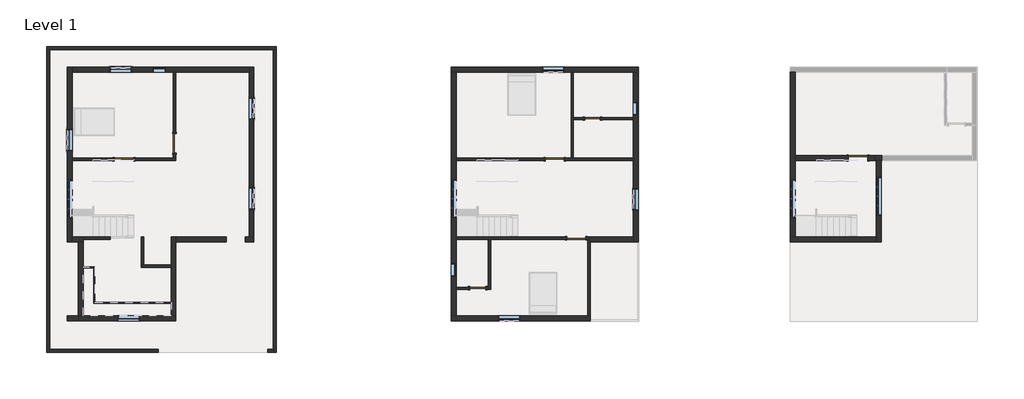
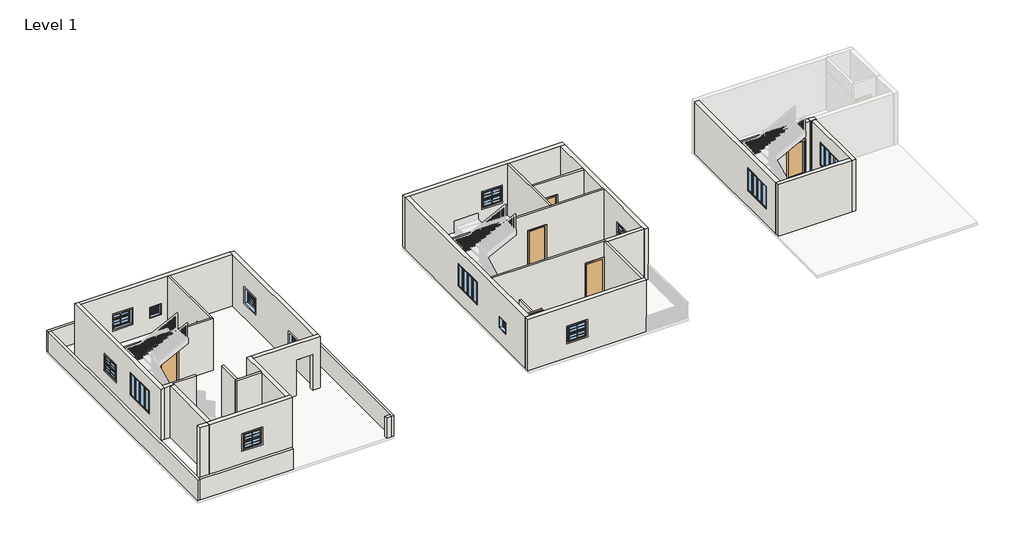
# One storey, part 1 of 8: 40 walls, 15 windows, 7 doors.
"""IFC4 building model written with IfcOpenShell, lengths in millimetres."""

from ifc_helpers import new_model, si_unit, frame, origin, origin_with_axes, place, context, project, spatial, polyline, outline, extrude, faceted_brep, transform, mapped, element, save
from components import door_f2b275c1, door_d8f5dbb5, single_flush_door_3_17d80c48, single_flush_door_3_5e62189b, single_flush_door_3_89fc3733, window_fa0038f5, window_5487fb6d, window_f2d8fef0

model = new_model("IFC4")

# Units and contexts
model_context = context("Model", 3, world=origin())
ifc_project = project(units=[si_unit("LENGTHUNIT", "METRE", prefix="MILLI")], contexts=[model_context])

# Site, building, storey
site = spatial("IfcSite", under=ifc_project)
building = spatial("IfcBuilding", under=site)
storey = spatial("IfcBuildingStorey", under=building, Name="Level 1", Elevation=0.0)

# Doors
placement = place(None, origin())
door_shape = door_f2b275c1(model_context)
element("IfcDoor", 1, ObjectType="Single-Flush : door 2'6\"", at=placement, inside=storey, context=model_context, shape_type="MappedRepresentation", body=[
    mapped(door_shape, transform((2134.2191518, 4539.4100713, 0.0), x_axis=(-1.0, 0.0, 0.0), y_axis=(0.0, -1.0, 0.0), z_axis=(0.0, 0.0, 1.0))),
])
door_2_shape = door_d8f5dbb5(model_context)
element("IfcDoor", 2, ObjectType="Single-Flush : door 2'6\"", at=placement, inside=storey, context=model_context, shape_type="MappedRepresentation", body=[
    mapped(door_2_shape, transform((-3352.1808482, -3575.8899287, 0.0), x_axis=(1.0, 0.0, 0.0), y_axis=(0.0, 1.0, 0.0), z_axis=(0.0, 0.0, 1.0))),
])
single_flush_door_3_shape = single_flush_door_3_17d80c48(model_context)
element("IfcDoor", 3, ObjectType="Single-Flush : door 3'", at=placement, inside=storey, context=model_context, shape_type="MappedRepresentation", body=[
    mapped(single_flush_door_3_shape, transform((-20233.4289184, 2596.3100713, 0.0), x_axis=(1.0, 0.0, 0.0), y_axis=(0.0, 1.0, 0.0), z_axis=(0.0, 0.0, 1.0))),
])
element("IfcDoor", 4, ObjectType="Single-Flush : door 3'", at=placement, inside=storey, context=model_context, shape_type="MappedRepresentation", body=[
    mapped(single_flush_door_3_shape, transform((330.8191518, 2596.3100713, 0.0), x_axis=(1.0, 0.0, 0.0), y_axis=(0.0, 1.0, 0.0), z_axis=(0.0, 0.0, 1.0))),
])
single_flush_door_3_2_shape = single_flush_door_3_5e62189b(model_context)
element("IfcDoor", 5, ObjectType="Single-Flush : door 3'", at=placement, inside=storey, context=model_context, shape_type="MappedRepresentation", body=[
    mapped(single_flush_door_3_2_shape, transform((-17820.4289184, 3358.3100713, 0.0), x_axis=(0.0, -1.0, 0.0), y_axis=(1.0, 0.0, 0.0), z_axis=(0.0, 0.0, 1.0))),
])
element("IfcDoor", 6, ObjectType="Single-Flush : door 3'", at=placement, inside=storey, context=model_context, shape_type="MappedRepresentation", body=[
    mapped(single_flush_door_3_2_shape, transform((1359.5191518, -1175.5899287, 0.0), x_axis=(1.0, 0.0, 0.0), y_axis=(0.0, 1.0, 0.0), z_axis=(0.0, 0.0, 1.0))),
])
single_flush_door_3_3_shape = single_flush_door_3_89fc3733(model_context)
element("IfcDoor", 7, ObjectType="Single-Flush : door 3'", at=placement, inside=storey, context=model_context, shape_type="MappedRepresentation", body=[
    mapped(single_flush_door_3_3_shape, transform((14813.742447, 2653.4600713, 0.0), x_axis=(1.0, 0.0, 0.0), y_axis=(0.0, 1.0, 0.0), z_axis=(0.0, 0.0, 1.0))),
])

# Walls
element("IfcWall", 8, at=placement, inside=storey, context=model_context, shape_type="Brep", body=[
    faceted_brep([(-23935.4789184, 7835.0600713, 0.0), (-23783.0789184, 7835.0600713, 0.0), (-13115.0789184, 7835.0600713, 0.0), (-12962.6789184, 7835.0600713, 0.0), (-12962.6789184, 7835.0600713, 1219.2), (-13115.0789184, 7835.0600713, 1219.2), (-23783.0789184, 7835.0600713, 1219.2), (-23935.4789184, 7835.0600713, 1219.2), (-23935.4789184, 7987.4600713, 0.0), (-23935.4789184, 7987.4600713, 1219.2), (-12962.6789184, 7987.4600713, 1219.2), (-12962.6789184, 7987.4600713, 0.0)], [[[0, 1, 2, 3, 4, 5, 6, 7]], [[8, 9, 10, 11]], [[3, 2, 1, 0, 8, 11]], [[7, 6, 5, 4, 10, 9]], [[4, 3, 11, 10]], [[0, 7, 9, 8]]]),
])
element("IfcWall", 9, at=placement, inside=storey, context=model_context, shape_type="Brep", body=[
    faceted_brep([(-13115.0789184, 7835.0600713, 0.0), (-13115.0789184, -6490.5399287, 0.0), (-13115.0789184, -6642.9399287, 0.0), (-13115.0789184, -6642.9399287, 1219.2), (-13115.0789184, -6490.5399287, 1219.2), (-13115.0789184, 7835.0600713, 1219.2), (-12962.6789184, 7835.0600713, 0.0), (-12962.6789184, 7835.0600713, 1219.2), (-12962.6789184, -6642.9399287, 1219.2), (-12962.6789184, -6642.9399287, 0.0)], [[[0, 1, 2, 3, 4, 5]], [[6, 7, 8, 9]], [[2, 1, 0, 6, 9]], [[5, 4, 3, 8, 7]], [[0, 5, 7, 6]], [[3, 2, 9, 8]]]),
])
element("IfcWall", 10, at=placement, inside=storey, context=model_context, shape_type="Brep", body=[
    faceted_brep([(-23935.4789184, 7835.0600713, 0.0), (-23935.4789184, -6642.9399287, 0.0), (-23935.4789184, -6642.9399287, 1219.2), (-23935.4789184, 7835.0600713, 1219.2), (-23783.0789184, 7835.0600713, 0.0), (-23783.0789184, 7835.0600713, 1219.2), (-23783.0789184, -6490.5399287, 1219.2), (-23783.0789184, -6642.9399287, 1219.2), (-23783.0789184, -6642.9399287, 0.0), (-23783.0789184, -6490.5399287, 0.0)], [[[0, 1, 2, 3]], [[4, 5, 6, 7, 8, 9]], [[1, 0, 4, 9, 8]], [[3, 2, 7, 6, 5]], [[0, 3, 5, 4]], [[2, 1, 8, 7]]]),
])
element("IfcWall", 11, at=placement, inside=storey, context=model_context, shape_type="SweptSolid", body=[
    extrude(outline(polyline([(-18601.4789184, -6642.9399287), (-23783.0789184, -6642.9399287), (-23783.0789184, -6490.5399287), (-18601.4789184, -6490.5399287), (-18601.4789184, -6642.9399287)])), origin_with_axes(), (0.0, 0.0, 1.0), 1219.2),
])
element("IfcWall", 12, at=placement, inside=storey, context=model_context, shape_type="SweptSolid", body=[
    extrude(outline(polyline([(-13115.0789184, -6642.9399287), (-13376.8812127, -6642.9399287), (-13376.8812127, -6490.5399287), (-13115.0789184, -6490.5399287), (-13115.0789184, -6642.9399287)])), origin_with_axes(), (0.0, 0.0, 1.0), 1219.2),
])
element("IfcWall", 13, ObjectType="W 2\"", at=placement, inside=storey, context=model_context, shape_type="Brep", body=[
    faceted_brep([(-22182.8789184, -2591.6399287, 0.0), (-21674.8789184, -2591.6399287, 0.0), (-21624.0789184, -2591.6399287, 0.0), (-21624.0789184, -2591.6399287, 1524.0), (-21674.8789184, -2591.6399287, 1524.0), (-22182.8789184, -2591.6399287, 1524.0), (-22182.8789184, -2540.8399287, 0.0), (-22182.8789184, -2540.8399287, 1524.0), (-21624.0789184, -2540.8399287, 1524.0), (-21624.0789184, -2540.8399287, 0.0)], [[[0, 1, 2, 3, 4, 5]], [[6, 7, 8, 9]], [[2, 1, 0, 6, 9]], [[5, 4, 3, 8, 7]], [[0, 5, 7, 6]], [[3, 2, 9, 8]]]),
])
element("IfcWall", 14, ObjectType="W 2\"", at=placement, inside=storey, context=model_context, shape_type="Brep", body=[
    faceted_brep([(-21674.8789184, -2591.6399287, 0.0), (-21674.8789184, -4306.1399287, 0.0), (-21674.8789184, -4306.1399287, 1524.0), (-21674.8789184, -2591.6399287, 1524.0), (-21624.0789184, -2591.6399287, 0.0), (-21624.0789184, -2591.6399287, 1524.0), (-21624.0789184, -4255.3399287, 1524.0), (-21624.0789184, -4306.1399287, 1524.0), (-21624.0789184, -4306.1399287, 0.0), (-21624.0789184, -4255.3399287, 0.0)], [[[0, 1, 2, 3]], [[4, 5, 6, 7, 8, 9]], [[1, 0, 4, 9, 8]], [[3, 2, 7, 6, 5]], [[0, 3, 5, 4]], [[2, 1, 8, 7]]]),
])
element("IfcWall", 15, ObjectType="W 2\"", at=placement, inside=storey, context=model_context, shape_type="SweptSolid", body=[
    extrude(outline(polyline([(-17991.8789184, -4306.1399287), (-21624.0789184, -4306.1399287), (-21624.0789184, -4255.3399287), (-17991.8789184, -4255.3399287), (-17991.8789184, -4306.1399287)])), origin_with_axes(), (0.0, 0.0, 1.0), 1524.0),
])
element("IfcWall", 16, ObjectType="WALL 4.5\"", at=placement, inside=storey, context=model_context, shape_type="Brep", body=[
    faceted_brep([(-19776.2289184, 2539.1600713, 2032.0), (-19776.2289184, 2539.1600713, 0.0), (-17763.2789184, 2539.1600713, 0.0), (-17763.2789184, 2539.1600713, 3048.0), (-22716.2789184, 2539.1600713, 3048.0), (-22716.2789184, 2539.1600713, 0.0), (-20690.6289184, 2539.1600713, 0.0), (-20690.6289184, 2539.1600713, 2032.0), (-17763.2789184, 2653.4600713, 0.0), (-17877.5789184, 2653.4600713, 0.0), (-19776.2289184, 2653.4600713, 0.0), (-19776.2289184, 2653.4600713, 2032.0), (-20690.6289184, 2653.4600713, 2032.0), (-20690.6289184, 2653.4600713, 0.0), (-22716.2789184, 2653.4600713, 0.0), (-22716.2789184, 2653.4600713, 3048.0), (-17877.5789184, 2653.4600713, 3048.0), (-17763.2789184, 2653.4600713, 3048.0)], [[[0, 1, 2, 3, 4, 5, 6, 7]], [[8, 9, 10, 11, 12, 13, 14, 15, 16, 17]], [[6, 5, 14, 13]], [[2, 1, 10, 9, 8]], [[4, 3, 17, 16, 15]], [[5, 4, 15, 14]], [[3, 2, 8, 17]], [[11, 10, 1, 0]], [[12, 11, 0, 7]], [[13, 12, 7, 6]]]),
])
element("IfcWall", 17, ObjectType="WALL 4.5\"", at=placement, inside=storey, context=model_context, shape_type="SweptSolid", body=[
    extrude(outline(polyline([(2901.1100713, 2032.0), (2901.1100713, 0.0), (2653.4600713, 0.0), (2653.4600713, 3048.0), (6768.2600713, 3048.0), (6768.2600713, 0.0), (3815.5100713, 0.0), (3815.5100713, 2032.0), (2901.1100713, 2032.0)])), frame((-17877.5789184, 0.0, 0.0), z_axis=(1.0, 0.0, 0.0), x_axis=(0.0, 1.0, 0.0)), (0.0, 0.0, 1.0), 114.3),
])
element("IfcWall", 18, ObjectType="WALL 4.5\"", at=placement, inside=storey, context=model_context, shape_type="SweptSolid", body=[
    extrude(outline(polyline([(-20887.4789184, -1232.7399287), (-22182.8789184, -1232.7399287), (-22182.8789184, -1118.4399287), (-20887.4789184, -1118.4399287), (-20887.4789184, -1232.7399287)])), origin_with_axes(), (0.0, 0.0, 1.0), 3048.0),
])
element("IfcWall", 19, ObjectType="WALL 4.5\"", at=placement, inside=storey, context=model_context, shape_type="Brep", body=[
    faceted_brep([(-17991.8789184, -2451.9399287, 0.0), (-19287.2789184, -2451.9399287, 0.0), (-19401.5789184, -2451.9399287, 0.0), (-19401.5789184, -2451.9399287, 3048.0), (-19287.2789184, -2451.9399287, 3048.0), (-17991.8789184, -2451.9399287, 3048.0), (-17991.8789184, -2566.2399287, 0.0), (-17991.8789184, -2566.2399287, 3048.0), (-19401.5789184, -2566.2399287, 3048.0), (-19401.5789184, -2566.2399287, 0.0)], [[[0, 1, 2, 3, 4, 5]], [[6, 7, 8, 9]], [[2, 1, 0, 6, 9]], [[5, 4, 3, 8, 7]], [[0, 5, 7, 6]], [[3, 2, 9, 8]]]),
])
element("IfcWall", 20, ObjectType="WALL 4.5\"", at=placement, inside=storey, context=model_context, shape_type="SweptSolid", body=[
    extrude(outline(polyline([(-19287.2789184, -1118.4399287), (-19287.2789184, -2451.9399287), (-19401.5789184, -2451.9399287), (-19401.5789184, -1118.4399287), (-19287.2789184, -1118.4399287)])), origin_with_axes(), (0.0, 0.0, 1.0), 3048.0),
])
element("IfcWall", 21, ObjectType="WALL 4.5\"", at=placement, inside=storey, context=model_context, shape_type="Brep", body=[
    faceted_brep([(1969.1191518, -1118.4399287, 0.0), (1816.7191518, -1118.4399287, 0.0), (1816.7191518, -1118.4399287, 2032.0), (902.3191518, -1118.4399287, 2032.0), (902.3191518, -1118.4399287, 0.0), (-4374.5308482, -1118.4399287, 0.0), (-4374.5308482, -1118.4399287, 3048.0), (1969.1191518, -1118.4399287, 3048.0), (1816.7191518, -1232.7399287, 2032.0), (1816.7191518, -1232.7399287, 0.0), (1911.9691518, -1232.7399287, 0.0), (1969.1191518, -1232.7399287, 0.0), (1969.1191518, -1232.7399287, 3048.0), (1911.9691518, -1232.7399287, 3048.0), (-4374.5308482, -1232.7399287, 3048.0), (-4374.5308482, -1232.7399287, 0.0), (-2850.5308482, -1232.7399287, 0.0), (-2736.2308482, -1232.7399287, 0.0), (902.3191518, -1232.7399287, 0.0), (902.3191518, -1232.7399287, 2032.0)], [[[0, 1, 2, 3, 4, 5, 6, 7]], [[8, 9, 10, 11, 12, 13, 14, 15, 16, 17, 18, 19]], [[11, 10, 9, 1, 0]], [[18, 17, 16, 15, 5, 4]], [[7, 6, 14, 13, 12]], [[0, 7, 12, 11]], [[6, 5, 15, 14]], [[2, 1, 9, 8]], [[3, 2, 8, 19]], [[4, 3, 19, 18]]]),
])
element("IfcWall", 22, ObjectType="WALL 4.5\"", at=placement, inside=storey, context=model_context, shape_type="Brep", body=[
    faceted_brep([(4083.6691518, 2653.4600713, 0.0), (1226.1691518, 2653.4600713, 0.0), (1111.8691518, 2653.4600713, 0.0), (788.0191518, 2653.4600713, 0.0), (788.0191518, 2653.4600713, 2032.0), (-126.3808482, 2653.4600713, 2032.0), (-126.3808482, 2653.4600713, 0.0), (-4374.5308482, 2653.4600713, 0.0), (-4374.5308482, 2653.4600713, 3048.0), (1111.8691518, 2653.4600713, 3048.0), (1226.1691518, 2653.4600713, 3048.0), (4083.6691518, 2653.4600713, 3048.0), (788.0191518, 2539.1600713, 2032.0), (788.0191518, 2539.1600713, 0.0), (4083.6691518, 2539.1600713, 0.0), (4083.6691518, 2539.1600713, 3048.0), (-4374.5308482, 2539.1600713, 3048.0), (-4374.5308482, 2539.1600713, 0.0), (-126.3808482, 2539.1600713, 0.0), (-126.3808482, 2539.1600713, 2032.0)], [[[0, 1, 2, 3, 4, 5, 6, 7, 8, 9, 10, 11]], [[12, 13, 14, 15, 16, 17, 18, 19]], [[18, 17, 7, 6]], [[14, 13, 3, 2, 1, 0]], [[11, 10, 9, 8, 16, 15]], [[0, 11, 15, 14]], [[8, 7, 17, 16]], [[4, 3, 13, 12]], [[5, 4, 12, 19]], [[6, 5, 19, 18]]]),
])
element("IfcWall", 23, ObjectType="WALL 4.5\"", at=placement, inside=storey, context=model_context, shape_type="Brep", body=[
    faceted_brep([(1111.8691518, 6768.2600713, 0.0), (1111.8691518, 2653.4600713, 0.0), (1111.8691518, 2653.4600713, 3048.0), (1111.8691518, 6768.2600713, 3048.0), (1226.1691518, 6768.2600713, 0.0), (1226.1691518, 6768.2600713, 3048.0), (1226.1691518, 4596.5600713, 3048.0), (1226.1691518, 4482.2600713, 3048.0), (1226.1691518, 2653.4600713, 3048.0), (1226.1691518, 2653.4600713, 0.0), (1226.1691518, 4482.2600713, 0.0), (1226.1691518, 4596.5600713, 0.0)], [[[0, 1, 2, 3]], [[4, 5, 6, 7, 8, 9, 10, 11]], [[1, 0, 4, 11, 10, 9]], [[3, 2, 8, 7, 6, 5]], [[0, 3, 5, 4]], [[2, 1, 9, 8]]]),
])
element("IfcWall", 24, ObjectType="WALL 4.5\"", at=placement, inside=storey, context=model_context, shape_type="SweptSolid", body=[
    extrude(outline(polyline([(0.0, 1226.1691518), (0.0, 1753.2191518), (2032.0, 1753.2191518), (2032.0, 2515.2191518), (0.0, 2515.2191518), (0.0, 4083.6691518), (3048.0, 4083.6691518), (3048.0, 1226.1691518), (0.0, 1226.1691518)])), frame((0.0, 4482.2600713, 0.0), z_axis=(0.0, 1.0, 0.0), x_axis=(0.0, 0.0, 1.0)), (0.0, 0.0, 1.0), 114.3),
])
element("IfcWall", 25, ObjectType="WALL 4.5\"", at=placement, inside=storey, context=model_context, shape_type="SweptSolid", body=[
    extrude(outline(polyline([(2026.2691518, -1347.0399287), (2026.2691518, -4890.3399287), (1911.9691518, -4890.3399287), (1911.9691518, -1232.7399287), (1969.1191518, -1232.7399287), (1969.1191518, -1347.0399287), (2026.2691518, -1347.0399287)])), origin_with_axes(), (0.0, 0.0, 1.0), 3048.0),
])
element("IfcWall", 26, ObjectType="WALL 4.5\"", at=placement, inside=storey, context=model_context, shape_type="Brep", body=[
    faceted_brep([(-2850.5308482, -1232.7399287, 0.0), (-2850.5308482, -3518.7399287, 0.0), (-2850.5308482, -3633.0399287, 0.0), (-2850.5308482, -3633.0399287, 1219.2), (-2850.5308482, -3518.7399287, 1219.2), (-2850.5308482, -1232.7399287, 1219.2), (-2736.2308482, -1232.7399287, 0.0), (-2736.2308482, -1232.7399287, 1219.2), (-2736.2308482, -3633.0399287, 1219.2), (-2736.2308482, -3633.0399287, 0.0)], [[[0, 1, 2, 3, 4, 5]], [[6, 7, 8, 9]], [[2, 1, 0, 6, 9]], [[5, 4, 3, 8, 7]], [[0, 5, 7, 6]], [[3, 2, 9, 8]]]),
])
element("IfcWall", 27, ObjectType="WALL 4.5\"", at=placement, inside=storey, context=model_context, shape_type="SweptSolid", body=[
    extrude(outline(polyline([(-2850.5308482, -3518.7399287), (-2850.5308482, -3633.0399287), (-2971.1808482, -3633.0399287), (-2971.1808482, -3518.7399287), (-2850.5308482, -3518.7399287)])), origin_with_axes(), (0.0, 0.0, 1.0), 1219.2),
    extrude(outline(polyline([(-4374.5308482, -3633.0399287), (-4374.5308482, -3518.7399287), (-3733.1808482, -3518.7399287), (-3733.1808482, -3633.0399287), (-4374.5308482, -3633.0399287)])), origin_with_axes(), (0.0, 0.0, 1.0), 1219.2),
])
element("IfcWall", 28, ObjectType="WALL 9\"", at=placement, inside=storey, context=model_context, shape_type="Brep", body=[
    faceted_brep([(-22944.8789184, 6996.8600713, 0.0), (-22944.8789184, -1347.0399287, 0.0), (-22944.8789184, -1347.0399287, 3048.0), (-22944.8789184, 6996.8600713, 3048.0), (-22944.8789184, 1596.1850713, 2260.6), (-22944.8789184, -232.6149287, 2260.6), (-22944.8789184, -232.6149287, 914.4), (-22944.8789184, 1596.1850713, 914.4), (-22944.8789184, 4031.4100713, 1828.8), (-22944.8789184, 2990.0100713, 1828.8), (-22944.8789184, 2990.0100713, 914.4), (-22944.8789184, 4031.4100713, 914.4), (-22716.2789184, 6996.8600713, 0.0), (-22716.2789184, 6996.8600713, 3048.0), (-22716.2789184, 6768.2600713, 3048.0), (-22716.2789184, 2653.4600713, 3048.0), (-22716.2789184, 2539.1600713, 3048.0), (-22716.2789184, -1118.4399287, 3048.0), (-22716.2789184, -1347.0399287, 3048.0), (-22716.2789184, -1347.0399287, 0.0), (-22716.2789184, -1118.4399287, 0.0), (-22716.2789184, 2539.1600713, 0.0), (-22716.2789184, 2653.4600713, 0.0), (-22716.2789184, 6768.2600713, 0.0), (-22716.2789184, 1596.1850713, 2260.6), (-22716.2789184, 1596.1850713, 914.4), (-22716.2789184, -232.6149287, 914.4), (-22716.2789184, -232.6149287, 2260.6), (-22716.2789184, 4031.4100713, 1828.8), (-22716.2789184, 4031.4100713, 914.4), (-22716.2789184, 2990.0100713, 914.4), (-22716.2789184, 2990.0100713, 1828.8)], [[[0, 1, 2, 3], [4, 5, 6, 7], [8, 9, 10, 11]], [[12, 13, 14, 15, 16, 17, 18, 19, 20, 21, 22, 23], [24, 25, 26, 27], [28, 29, 30, 31]], [[1, 0, 12, 23, 22, 21, 20, 19]], [[3, 2, 18, 17, 16, 15, 14, 13]], [[2, 1, 19, 18]], [[0, 3, 13, 12]], [[25, 24, 4, 7]], [[26, 25, 7, 6]], [[27, 26, 6, 5]], [[24, 27, 5, 4]], [[29, 28, 8, 11]], [[30, 29, 11, 10]], [[31, 30, 10, 9]], [[28, 31, 9, 8]]]),
])
element("IfcWall", 29, ObjectType="WALL 9\"", at=placement, inside=storey, context=model_context, shape_type="Brep", body=[
    faceted_brep([(-22716.2789184, -1347.0399287, 0.0), (-22411.4789184, -1347.0399287, 0.0), (-22182.8789184, -1347.0399287, 0.0), (-22182.8789184, -1347.0399287, 3048.0), (-22411.4789184, -1347.0399287, 3048.0), (-22716.2789184, -1347.0399287, 3048.0), (-22716.2789184, -1118.4399287, 0.0), (-22716.2789184, -1118.4399287, 3048.0), (-22182.8789184, -1118.4399287, 3048.0), (-22182.8789184, -1118.4399287, 0.0), (-22182.8789184, -1232.7399287, 0.0), (-22182.8789184, -1232.7399287, 3048.0)], [[[0, 1, 2, 3, 4, 5]], [[6, 7, 8, 9]], [[2, 1, 0, 6, 9, 10]], [[5, 4, 3, 11, 8, 7]], [[0, 5, 7, 6]], [[3, 2, 10, 9, 8, 11]]]),
])
element("IfcWall", 30, ObjectType="WALL 9\"", at=placement, inside=storey, context=model_context, shape_type="Brep", body=[
    faceted_brep([(-22411.4789184, -1347.0399287, 0.0), (-22411.4789184, -4890.3399287, 0.0), (-22411.4789184, -4890.3399287, 3048.0), (-22411.4789184, -1347.0399287, 3048.0), (-22182.8789184, -1347.0399287, 0.0), (-22182.8789184, -1347.0399287, 3048.0), (-22182.8789184, -4890.3399287, 3048.0), (-22182.8789184, -4890.3399287, 0.0), (-22182.8789184, -2591.6399287, 0.0), (-22182.8789184, -2540.8399287, 0.0)], [[[0, 1, 2, 3]], [[4, 5, 6, 7, 8, 9]], [[1, 0, 4, 9, 8, 7]], [[3, 2, 6, 5]], [[0, 3, 5, 4]], [[2, 1, 7, 6]]]),
])
element("IfcWall", 31, ObjectType="WALL 9\"", at=placement, inside=storey, context=model_context, shape_type="SweptSolid", body=[
    extrude(outline(polyline([(-22417.8289184, -5118.9399287), (-22944.8789184, -5118.9399287), (-22944.8789184, -4890.3399287), (-22417.8289184, -4890.3399287), (-22417.8289184, -5118.9399287)])), origin_with_axes(), (0.0, 0.0, 1.0), 3048.0),
])
element("IfcWall", 32, ObjectType="WALL 9\"", at=placement, inside=storey, context=model_context, shape_type="Brep", body=[
    faceted_brep([(-17763.2789184, -4890.3399287, 0.0), (-17763.2789184, -1347.0399287, 0.0), (-17763.2789184, -1118.4399287, 0.0), (-17763.2789184, -1118.4399287, 3048.0), (-17763.2789184, -1347.0399287, 3048.0), (-17763.2789184, -4890.3399287, 3048.0), (-17991.8789184, -4890.3399287, 0.0), (-17991.8789184, -4890.3399287, 3048.0), (-17991.8789184, -2566.2399287, 3048.0), (-17991.8789184, -2451.9399287, 3048.0), (-17991.8789184, -1118.4399287, 3048.0), (-17991.8789184, -1118.4399287, 0.0), (-17991.8789184, -2451.9399287, 0.0), (-17991.8789184, -2566.2399287, 0.0), (-17991.8789184, -4255.3399287, 0.0), (-17991.8789184, -4306.1399287, 0.0)], [[[0, 1, 2, 3, 4, 5]], [[6, 7, 8, 9, 10, 11, 12, 13, 14, 15]], [[2, 1, 0, 6, 15, 14, 13, 12, 11]], [[5, 4, 3, 10, 9, 8, 7]], [[0, 5, 7, 6]], [[3, 2, 11, 10]]]),
])
element("IfcWall", 33, ObjectType="WALL 9\"", at=placement, inside=storey, context=model_context, shape_type="Brep", body=[
    faceted_brep([(-14029.4789184, -1347.0399287, 3048.0), (-17763.2789184, -1347.0399287, 3048.0), (-17763.2789184, -1347.0399287, 0.0), (-15362.9789184, -1347.0399287, 0.0), (-15362.9789184, -1347.0399287, 2133.6), (-14448.5789184, -1347.0399287, 2133.6), (-14448.5789184, -1347.0399287, 0.0), (-14029.4789184, -1347.0399287, 0.0), (-17763.2789184, -1118.4399287, 3048.0), (-14258.0789184, -1118.4399287, 3048.0), (-14029.4789184, -1118.4399287, 3048.0), (-14029.4789184, -1118.4399287, 0.0), (-14258.0789184, -1118.4399287, 0.0), (-14448.5789184, -1118.4399287, 0.0), (-14448.5789184, -1118.4399287, 2133.6), (-15362.9789184, -1118.4399287, 2133.6), (-15362.9789184, -1118.4399287, 0.0), (-17763.2789184, -1118.4399287, 0.0)], [[[0, 1, 2, 3, 4, 5, 6, 7]], [[8, 9, 10, 11, 12, 13, 14, 15, 16, 17]], [[2, 17, 16, 3]], [[11, 7, 6, 13, 12]], [[1, 0, 10, 9, 8]], [[2, 1, 8, 17]], [[0, 7, 11, 10]], [[5, 14, 13, 6]], [[14, 5, 4, 15]], [[15, 4, 3, 16]]]),
])
element("IfcWall", 34, ObjectType="WALL 9\"", at=placement, inside=storey, context=model_context, shape_type="Brep", body=[
    faceted_brep([(-14029.4789184, -1118.4399287, 0.0), (-14029.4789184, 6996.8600713, 0.0), (-14029.4789184, 6996.8600713, 3048.0), (-14029.4789184, -1118.4399287, 3048.0), (-14029.4789184, 4507.6600713, 1828.8), (-14029.4789184, 5549.0600713, 1828.8), (-14029.4789184, 5549.0600713, 914.4), (-14029.4789184, 4507.6600713, 914.4), (-14029.4789184, 202.3600713, 1828.8), (-14029.4789184, 1243.7600713, 1828.8), (-14029.4789184, 1243.7600713, 914.4), (-14029.4789184, 202.3600713, 914.4), (-14258.0789184, -1118.4399287, 0.0), (-14258.0789184, -1118.4399287, 3048.0), (-14258.0789184, 6768.2600713, 3048.0), (-14258.0789184, 6996.8600713, 3048.0), (-14258.0789184, 6996.8600713, 0.0), (-14258.0789184, 6768.2600713, 0.0), (-14258.0789184, 4507.6600713, 1828.8), (-14258.0789184, 4507.6600713, 914.4), (-14258.0789184, 5549.0600713, 914.4), (-14258.0789184, 5549.0600713, 1828.8), (-14258.0789184, 202.3600713, 1828.8), (-14258.0789184, 202.3600713, 914.4), (-14258.0789184, 1243.7600713, 914.4), (-14258.0789184, 1243.7600713, 1828.8)], [[[0, 1, 2, 3], [4, 5, 6, 7], [8, 9, 10, 11]], [[12, 13, 14, 15, 16, 17], [18, 19, 20, 21], [22, 23, 24, 25]], [[1, 0, 12, 17, 16]], [[3, 2, 15, 14, 13]], [[0, 3, 13, 12]], [[2, 1, 16, 15]], [[19, 18, 4, 7]], [[20, 19, 7, 6]], [[21, 20, 6, 5]], [[18, 21, 5, 4]], [[23, 22, 8, 11]], [[24, 23, 11, 10]], [[25, 24, 10, 9]], [[22, 25, 9, 8]]]),
])
element("IfcWall", 35, ObjectType="WALL 9\"", at=placement, inside=storey, context=model_context, shape_type="Brep", body=[
    faceted_brep([(-14258.0789184, 6996.8600713, 0.0), (-22716.2789184, 6996.8600713, 0.0), (-22716.2789184, 6996.8600713, 3048.0), (-14258.0789184, 6996.8600713, 3048.0), (-19871.4789184, 6996.8600713, 1828.8), (-20912.8789184, 6996.8600713, 1828.8), (-20912.8789184, 6996.8600713, 914.4), (-19871.4789184, 6996.8600713, 914.4), (-18861.8289184, 6996.8600713, 1524.0), (-18861.8289184, 6996.8600713, 914.4), (-18252.2289184, 6996.8600713, 914.4), (-18252.2289184, 6996.8600713, 1524.0), (-14258.0789184, 6768.2600713, 0.0), (-14258.0789184, 6768.2600713, 3048.0), (-17763.2789184, 6768.2600713, 3048.0), (-17877.5789184, 6768.2600713, 3048.0), (-22716.2789184, 6768.2600713, 3048.0), (-22716.2789184, 6768.2600713, 0.0), (-17877.5789184, 6768.2600713, 0.0), (-17763.2789184, 6768.2600713, 0.0), (-19871.4789184, 6768.2600713, 1828.8), (-19871.4789184, 6768.2600713, 914.4), (-20912.8789184, 6768.2600713, 914.4), (-20912.8789184, 6768.2600713, 1828.8), (-18861.8289184, 6768.2600713, 1524.0), (-18252.2289184, 6768.2600713, 1524.0), (-18252.2289184, 6768.2600713, 914.4), (-18861.8289184, 6768.2600713, 914.4)], [[[0, 1, 2, 3], [4, 5, 6, 7], [8, 9, 10, 11]], [[12, 13, 14, 15, 16, 17, 18, 19], [20, 21, 22, 23], [24, 25, 26, 27]], [[1, 0, 12, 19, 18, 17]], [[3, 2, 16, 15, 14, 13]], [[0, 3, 13, 12]], [[2, 1, 17, 16]], [[21, 20, 4, 7]], [[22, 21, 7, 6]], [[23, 22, 6, 5]], [[20, 23, 5, 4]], [[9, 8, 24, 27]], [[10, 9, 27, 26]], [[11, 10, 26, 25]], [[8, 11, 25, 24]]]),
])
element("IfcWall", 36, ObjectType="WALL 9\"", at=placement, inside=storey, context=model_context, shape_type="Brep", body=[
    faceted_brep([(-4603.1308482, 6768.2600713, 0.0), (-4374.5308482, 6768.2600713, 0.0), (1111.8691518, 6768.2600713, 0.0), (1226.1691518, 6768.2600713, 0.0), (4083.6691518, 6768.2600713, 0.0), (4312.2691518, 6768.2600713, 0.0), (4312.2691518, 6768.2600713, 3048.0), (4083.6691518, 6768.2600713, 3048.0), (1226.1691518, 6768.2600713, 3048.0), (1111.8691518, 6768.2600713, 3048.0), (-4374.5308482, 6768.2600713, 3048.0), (-4603.1308482, 6768.2600713, 3048.0), (-266.0808482, 6768.2600713, 1828.8), (775.3191518, 6768.2600713, 1828.8), (775.3191518, 6768.2600713, 914.4), (-266.0808482, 6768.2600713, 914.4), (-4603.1308482, 6996.8600713, 0.0), (-4603.1308482, 6996.8600713, 3048.0), (4312.2691518, 6996.8600713, 3048.0), (4312.2691518, 6996.8600713, 0.0), (-266.0808482, 6996.8600713, 1828.8), (-266.0808482, 6996.8600713, 914.4), (775.3191518, 6996.8600713, 914.4), (775.3191518, 6996.8600713, 1828.8)], [[[0, 1, 2, 3, 4, 5, 6, 7, 8, 9, 10, 11], [12, 13, 14, 15]], [[16, 17, 18, 19], [20, 21, 22, 23]], [[5, 4, 3, 2, 1, 0, 16, 19]], [[11, 10, 9, 8, 7, 6, 18, 17]], [[6, 5, 19, 18]], [[0, 11, 17, 16]], [[21, 20, 12, 15]], [[22, 21, 15, 14]], [[23, 22, 14, 13]], [[20, 23, 13, 12]]]),
])
element("IfcWall", 37, ObjectType="WALL 9\"", at=placement, inside=storey, context=model_context, shape_type="Brep", body=[
    faceted_brep([(4083.6691518, 6768.2600713, 0.0), (4083.6691518, 4596.5600713, 0.0), (4083.6691518, 4482.2600713, 0.0), (4083.6691518, 2653.4600713, 0.0), (4083.6691518, 2539.1600713, 0.0), (4083.6691518, -1118.4399287, 0.0), (4083.6691518, -1347.0399287, 0.0), (4083.6691518, -1347.0399287, 3048.0), (4083.6691518, -1118.4399287, 3048.0), (4083.6691518, 2539.1600713, 3048.0), (4083.6691518, 2653.4600713, 3048.0), (4083.6691518, 4482.2600713, 3048.0), (4083.6691518, 4596.5600713, 3048.0), (4083.6691518, 6768.2600713, 3048.0), (4083.6691518, 1202.4850713, 1828.8), (4083.6691518, 161.0850713, 1828.8), (4083.6691518, 161.0850713, 914.4), (4083.6691518, 1202.4850713, 914.4), (4083.6691518, 5326.8100713, 1524.0), (4083.6691518, 4717.2100713, 1524.0), (4083.6691518, 4717.2100713, 914.4), (4083.6691518, 5326.8100713, 914.4), (4312.2691518, 6768.2600713, 0.0), (4312.2691518, 6768.2600713, 3048.0), (4312.2691518, -1347.0399287, 3048.0), (4312.2691518, -1347.0399287, 0.0), (4312.2691518, 1202.4850713, 1828.8), (4312.2691518, 1202.4850713, 914.4), (4312.2691518, 161.0850713, 914.4), (4312.2691518, 161.0850713, 1828.8), (4312.2691518, 5326.8100713, 1524.0), (4312.2691518, 5326.8100713, 914.4), (4312.2691518, 4717.2100713, 914.4), (4312.2691518, 4717.2100713, 1524.0)], [[[0, 1, 2, 3, 4, 5, 6, 7, 8, 9, 10, 11, 12, 13], [14, 15, 16, 17], [18, 19, 20, 21]], [[22, 23, 24, 25], [26, 27, 28, 29], [30, 31, 32, 33]], [[6, 5, 4, 3, 2, 1, 0, 22, 25]], [[13, 12, 11, 10, 9, 8, 7, 24, 23]], [[0, 13, 23, 22]], [[7, 6, 25, 24]], [[27, 26, 14, 17]], [[28, 27, 17, 16]], [[29, 28, 16, 15]], [[26, 29, 15, 14]], [[31, 30, 18, 21]], [[32, 31, 21, 20]], [[33, 32, 20, 19]], [[30, 33, 19, 18]]]),
])
element("IfcWall", 38, ObjectType="WALL 9\"", at=placement, inside=storey, context=model_context, shape_type="Brep", body=[
    faceted_brep([(4083.6691518, -1118.4399287, 0.0), (1969.1191518, -1118.4399287, 0.0), (1969.1191518, -1118.4399287, 3048.0), (4083.6691518, -1118.4399287, 3048.0), (4083.6691518, -1347.0399287, 0.0), (4083.6691518, -1347.0399287, 3048.0), (2026.2691518, -1347.0399287, 3048.0), (1969.1191518, -1347.0399287, 3048.0), (1969.1191518, -1347.0399287, 0.0), (2026.2691518, -1347.0399287, 0.0), (1969.1191518, -1232.7399287, 0.0), (1969.1191518, -1232.7399287, 3048.0)], [[[0, 1, 2, 3]], [[4, 5, 6, 7, 8, 9]], [[1, 0, 4, 9, 8, 10]], [[2, 1, 10, 8, 7, 11]], [[3, 2, 11, 7, 6, 5]], [[0, 3, 5, 4]]]),
])
element("IfcWall", 39, ObjectType="WALL 9\"", at=placement, inside=storey, context=model_context, shape_type="Brep", body=[
    faceted_brep([(2026.2691518, -4890.3399287, 0.0), (1911.9691518, -4890.3399287, 0.0), (-4374.5308482, -4890.3399287, 0.0), (-4603.1308482, -4890.3399287, 0.0), (-4603.1308482, -4890.3399287, 3048.0), (-4374.5308482, -4890.3399287, 3048.0), (1911.9691518, -4890.3399287, 3048.0), (2026.2691518, -4890.3399287, 3048.0), (-2367.9308482, -4890.3399287, 1828.8), (-2367.9308482, -4890.3399287, 914.4), (-1326.5308482, -4890.3399287, 914.4), (-1326.5308482, -4890.3399287, 1828.8), (2026.2691518, -5118.9399287, 0.0), (2026.2691518, -5118.9399287, 3048.0), (-4603.1308482, -5118.9399287, 3048.0), (-4603.1308482, -5118.9399287, 0.0), (-2367.9308482, -5118.9399287, 1828.8), (-1326.5308482, -5118.9399287, 1828.8), (-1326.5308482, -5118.9399287, 914.4), (-2367.9308482, -5118.9399287, 914.4)], [[[0, 1, 2, 3, 4, 5, 6, 7], [8, 9, 10, 11]], [[12, 13, 14, 15], [16, 17, 18, 19]], [[3, 2, 1, 0, 12, 15]], [[7, 6, 5, 4, 14, 13]], [[4, 3, 15, 14]], [[0, 7, 13, 12]], [[9, 8, 16, 19]], [[10, 9, 19, 18]], [[11, 10, 18, 17]], [[8, 11, 17, 16]]]),
])
element("IfcWall", 40, ObjectType="WALL 9\"", at=placement, inside=storey, context=model_context, shape_type="Brep", body=[
    faceted_brep([(-4374.5308482, -4890.3399287, 0.0), (-4374.5308482, -3633.0399287, 0.0), (-4374.5308482, -3518.7399287, 0.0), (-4374.5308482, -1232.7399287, 0.0), (-4374.5308482, -1118.4399287, 0.0), (-4374.5308482, 2539.1600713, 0.0), (-4374.5308482, 2653.4600713, 0.0), (-4374.5308482, 6768.2600713, 0.0), (-4374.5308482, 6768.2600713, 3048.0), (-4374.5308482, 2653.4600713, 3048.0), (-4374.5308482, 2539.1600713, 3048.0), (-4374.5308482, -1118.4399287, 3048.0), (-4374.5308482, -1232.7399287, 3048.0), (-4374.5308482, -4890.3399287, 3048.0), (-4374.5308482, 1624.7600713, 2260.6), (-4374.5308482, 1624.7600713, 914.4), (-4374.5308482, -204.0399287, 914.4), (-4374.5308482, -204.0399287, 2260.6), (-4374.5308482, -2394.7899287, 1524.0), (-4374.5308482, -2394.7899287, 914.4), (-4374.5308482, -3004.3899287, 914.4), (-4374.5308482, -3004.3899287, 1524.0), (-4603.1308482, -4890.3399287, 0.0), (-4603.1308482, -4890.3399287, 3048.0), (-4603.1308482, 6768.2600713, 3048.0), (-4603.1308482, 6768.2600713, 0.0), (-4603.1308482, 1624.7600713, 2260.6), (-4603.1308482, -204.0399287, 2260.6), (-4603.1308482, -204.0399287, 914.4), (-4603.1308482, 1624.7600713, 914.4), (-4603.1308482, -2394.7899287, 1524.0), (-4603.1308482, -3004.3899287, 1524.0), (-4603.1308482, -3004.3899287, 914.4), (-4603.1308482, -2394.7899287, 914.4)], [[[0, 1, 2, 3, 4, 5, 6, 7, 8, 9, 10, 11, 12, 13], [14, 15, 16, 17], [18, 19, 20, 21]], [[22, 23, 24, 25], [26, 27, 28, 29], [30, 31, 32, 33]], [[7, 6, 5, 4, 3, 2, 1, 0, 22, 25]], [[13, 12, 11, 10, 9, 8, 24, 23]], [[0, 13, 23, 22]], [[8, 7, 25, 24]], [[15, 14, 26, 29]], [[16, 15, 29, 28]], [[17, 16, 28, 27]], [[14, 17, 27, 26]], [[19, 18, 30, 33]], [[20, 19, 33, 32]], [[21, 20, 32, 31]], [[18, 21, 31, 30]]]),
])
element("IfcWall", 41, ObjectType="WALL 9\"", at=placement, inside=storey, context=model_context, shape_type="SweptSolid", body=[
    extrude(outline(polyline([(15690.042447, 2526.4600713), (15690.042447, 2539.1600713), (15918.642447, 2539.1600713), (15918.642447, 2526.4600713), (15690.042447, 2526.4600713)])), origin_with_axes(), (0.0, 0.0, 1.0), 3048.0),
])
element("IfcWall", 42, ObjectType="WALL 9\"", at=placement, inside=storey, context=model_context, shape_type="Brep", body=[
    faceted_brep([(15690.042447, -1118.4399287, 0.0), (11803.842447, -1118.4399287, 0.0), (11575.242447, -1118.4399287, 0.0), (11575.242447, -1118.4399287, 3048.0), (11803.842447, -1118.4399287, 3048.0), (14750.242447, -1118.4399287, 3048.0), (15690.042447, -1118.4399287, 3048.0), (15690.042447, -1347.0399287, 0.0), (15690.042447, -1347.0399287, 3048.0), (11575.242447, -1347.0399287, 3048.0), (11575.242447, -1347.0399287, 0.0)], [[[0, 1, 2, 3, 4, 5, 6]], [[7, 8, 9, 10]], [[2, 1, 0, 7, 10]], [[0, 6, 8, 7]], [[3, 2, 10, 9]], [[6, 5, 4, 3, 9, 8]]]),
])
element("IfcWall", 43, ObjectType="WALL 9\"", at=placement, inside=storey, context=model_context, shape_type="Brep", body=[
    faceted_brep([(11803.842447, -1118.4399287, 0.0), (11803.842447, 2539.1600713, 0.0), (11803.842447, 2767.7600713, 0.0), (11803.842447, 6768.2600713, 0.0), (11803.842447, 6768.2600713, 3048.0), (11803.842447, 2767.7600713, 3048.0), (11803.842447, 2539.1600713, 3048.0), (11803.842447, -1118.4399287, 3048.0), (11803.842447, 1624.7600713, 2260.6), (11803.842447, 1624.7600713, 914.4), (11803.842447, -204.0399287, 914.4), (11803.842447, -204.0399287, 2260.6), (11575.242447, -1118.4399287, 0.0), (11575.242447, -1118.4399287, 3048.0), (11575.242447, 6768.2600713, 3048.0), (11575.242447, 6768.2600713, 0.0), (11575.242447, 1624.7600713, 2260.6), (11575.242447, -204.0399287, 2260.6), (11575.242447, -204.0399287, 914.4), (11575.242447, 1624.7600713, 914.4)], [[[0, 1, 2, 3, 4, 5, 6, 7], [8, 9, 10, 11]], [[12, 13, 14, 15], [16, 17, 18, 19]], [[3, 2, 1, 0, 12, 15]], [[0, 7, 13, 12]], [[4, 3, 15, 14]], [[7, 6, 5, 4, 14, 13]], [[9, 8, 16, 19]], [[10, 9, 19, 18]], [[11, 10, 18, 17]], [[8, 11, 17, 16]]]),
])
element("IfcWall", 44, ObjectType="WALL 9\"", at=placement, inside=storey, context=model_context, shape_type="Brep", body=[
    faceted_brep([(-22417.8289184, -5118.9399287, 0.0), (-17763.2789184, -5118.9399287, 0.0), (-17763.2789184, -5118.9399287, 3048.0), (-22417.8289184, -5118.9399287, 3048.0), (-20531.8789184, -5118.9399287, 1828.8), (-19490.4789184, -5118.9399287, 1828.8), (-19490.4789184, -5118.9399287, 914.4), (-20531.8789184, -5118.9399287, 914.4), (-22417.8289184, -4890.3399287, 0.0), (-22417.8289184, -4890.3399287, 3048.0), (-22411.4789184, -4890.3399287, 3048.0), (-22182.8789184, -4890.3399287, 3048.0), (-17991.8789184, -4890.3399287, 3048.0), (-17763.2789184, -4890.3399287, 3048.0), (-17763.2789184, -4890.3399287, 0.0), (-17991.8789184, -4890.3399287, 0.0), (-22182.8789184, -4890.3399287, 0.0), (-22411.4789184, -4890.3399287, 0.0), (-20531.8789184, -4890.3399287, 1828.8), (-20531.8789184, -4890.3399287, 914.4), (-19490.4789184, -4890.3399287, 914.4), (-19490.4789184, -4890.3399287, 1828.8)], [[[0, 1, 2, 3], [4, 5, 6, 7]], [[8, 9, 10, 11, 12, 13, 14, 15, 16, 17], [18, 19, 20, 21]], [[1, 0, 8, 17, 16, 15, 14]], [[3, 2, 13, 12, 11, 10, 9]], [[0, 3, 9, 8]], [[2, 1, 14, 13]], [[19, 18, 4, 7]], [[20, 19, 7, 6]], [[21, 20, 6, 5]], [[18, 21, 5, 4]]]),
])
element("IfcWall", 45, ObjectType="WALL 9\"", at=placement, inside=storey, context=model_context, shape_type="Brep", body=[
    faceted_brep([(15690.042447, 2526.4600713, 0.0), (15690.042447, -1118.4399287, 0.0), (15690.042447, -1347.0399287, 0.0), (15690.042447, -1347.0399287, 3048.0), (15690.042447, -1118.4399287, 3048.0), (15690.042447, 2526.4600713, 3048.0), (15690.042447, 1739.0600713, 2260.6), (15690.042447, -89.7399287, 2260.6), (15690.042447, -89.7399287, 914.4), (15690.042447, 1739.0600713, 914.4), (15918.642447, 2526.4600713, 0.0), (15918.642447, 2526.4600713, 3048.0), (15918.642447, -1347.0399287, 3048.0), (15918.642447, -1347.0399287, 0.0), (15918.642447, 1739.0600713, 2260.6), (15918.642447, 1739.0600713, 914.4), (15918.642447, -89.7399287, 914.4), (15918.642447, -89.7399287, 2260.6)], [[[0, 1, 2, 3, 4, 5], [6, 7, 8, 9]], [[10, 11, 12, 13], [14, 15, 16, 17]], [[2, 1, 0, 10, 13]], [[0, 5, 11, 10]], [[3, 2, 13, 12]], [[5, 4, 3, 12, 11]], [[14, 17, 7, 6]], [[17, 16, 8, 7]], [[16, 15, 9, 8]], [[15, 14, 6, 9]]]),
])
element("IfcWall", 46, ObjectType="WALL 9\"", at=placement, inside=storey, context=model_context, shape_type="Brep", body=[
    faceted_brep([(15956.742447, 2767.7600713, 0.0), (15601.142447, 2767.7600713, 0.0), (15601.142447, 2767.7600713, 3048.0), (15956.742447, 2767.7600713, 3048.0), (15956.742447, 2539.1600713, 0.0), (15956.742447, 2539.1600713, 3048.0), (15918.642447, 2539.1600713, 3048.0), (15690.042447, 2539.1600713, 3048.0), (15601.142447, 2539.1600713, 3048.0), (15601.142447, 2539.1600713, 0.0), (15690.042447, 2539.1600713, 0.0), (15918.642447, 2539.1600713, 0.0)], [[[0, 1, 2, 3]], [[4, 5, 6, 7, 8, 9, 10, 11]], [[1, 0, 4, 11, 10, 9]], [[2, 1, 9, 8]], [[0, 3, 5, 4]], [[3, 2, 8, 7, 6, 5]]]),
])
element("IfcWall", 47, ObjectType="WALL 9\"", at=placement, inside=storey, context=model_context, shape_type="Brep", body=[
    faceted_brep([(15601.142447, 2767.7600713, 0.0), (15270.942447, 2767.7600713, 0.0), (15270.942447, 2767.7600713, 2032.0), (14356.542447, 2767.7600713, 2032.0), (14356.542447, 2767.7600713, 0.0), (11803.842447, 2767.7600713, 0.0), (11803.842447, 2767.7600713, 3048.0), (15601.142447, 2767.7600713, 3048.0), (15270.942447, 2539.1600713, 2032.0), (15270.942447, 2539.1600713, 0.0), (15601.142447, 2539.1600713, 0.0), (15601.142447, 2539.1600713, 3048.0), (14750.242447, 2539.1600713, 3048.0), (11803.842447, 2539.1600713, 3048.0), (11803.842447, 2539.1600713, 0.0), (14356.542447, 2539.1600713, 0.0), (14356.542447, 2539.1600713, 2032.0)], [[[0, 1, 2, 3, 4, 5, 6, 7]], [[8, 9, 10, 11, 12, 13, 14, 15, 16]], [[15, 14, 5, 4]], [[10, 9, 1, 0]], [[0, 7, 11, 10]], [[6, 5, 14, 13]], [[7, 6, 13, 12, 11]], [[4, 3, 16, 15]], [[3, 2, 8, 16]], [[2, 1, 9, 8]]]),
])

# Windows
window_shape = window_fa0038f5(model_context)
element("IfcWindow", 48, ObjectType="Window-Awning-Double-Vertical : 41\" x 36\"", at=placement, inside=storey, context=model_context, shape_type="MappedRepresentation", body=[
    mapped(window_shape, transform((-22830.5789184, 3510.7100713, 0.0), x_axis=(0.0, 1.0, 0.0), y_axis=(-1.0, 0.0, 0.0), z_axis=(0.0, 0.0, 1.0))),
])
element("IfcWindow", 49, ObjectType="Window-Awning-Double-Vertical : 41\" x 36\"", at=placement, inside=storey, context=model_context, shape_type="MappedRepresentation", body=[
    mapped(window_shape, transform((-20392.1789184, 6882.5600713, 0.0), x_axis=(1.0, 0.0, 0.0), y_axis=(0.0, 1.0, 0.0), z_axis=(0.0, 0.0, 1.0))),
])
element("IfcWindow", 50, ObjectType="Window-Awning-Double-Vertical : 41\" x 36\"", at=placement, inside=storey, context=model_context, shape_type="MappedRepresentation", body=[
    mapped(window_shape, transform((-14143.7789184, 5028.3600713, 0.0), x_axis=(0.0, -1.0, 0.0), y_axis=(1.0, 0.0, 0.0), z_axis=(0.0, 0.0, 1.0))),
])
element("IfcWindow", 51, ObjectType="Window-Awning-Double-Vertical : 41\" x 36\"", at=placement, inside=storey, context=model_context, shape_type="MappedRepresentation", body=[
    mapped(window_shape, transform((-14143.7789184, 723.0600713, 0.0), x_axis=(0.0, -1.0, 0.0), y_axis=(1.0, 0.0, 0.0), z_axis=(0.0, 0.0, 1.0))),
])
element("IfcWindow", 52, ObjectType="Window-Awning-Double-Vertical : 41\" x 36\"", at=placement, inside=storey, context=model_context, shape_type="MappedRepresentation", body=[
    mapped(window_shape, transform((-20011.1789184, -5004.6399287, 0.0), x_axis=(-1.0, 0.0, 0.0), y_axis=(0.0, -1.0, 0.0), z_axis=(0.0, 0.0, 1.0))),
])
element("IfcWindow", 53, ObjectType="Window-Awning-Double-Vertical : 41\" x 36\"", at=placement, inside=storey, context=model_context, shape_type="MappedRepresentation", body=[
    mapped(window_shape, transform((-1847.2308482, -5004.6399287, 0.0), x_axis=(-1.0, 0.0, 0.0), y_axis=(0.0, -1.0, 0.0), z_axis=(0.0, 0.0, 1.0))),
])
element("IfcWindow", 54, ObjectType="Window-Awning-Double-Vertical : 41\" x 36\"", at=placement, inside=storey, context=model_context, shape_type="MappedRepresentation", body=[
    mapped(window_shape, transform((4197.9691518, 681.7850713, 0.0), x_axis=(0.0, 1.0, 0.0), y_axis=(-1.0, 0.0, 0.0), z_axis=(0.0, 0.0, 1.0))),
])
element("IfcWindow", 55, ObjectType="Window-Awning-Double-Vertical : 41\" x 36\"", at=placement, inside=storey, context=model_context, shape_type="MappedRepresentation", body=[
    mapped(window_shape, transform((254.6191518, 6882.5600713, 0.0), x_axis=(-1.0, 0.0, 0.0), y_axis=(0.0, -1.0, 0.0), z_axis=(0.0, 0.0, 1.0))),
])
window_2_shape = window_5487fb6d(model_context)
element("IfcWindow", 56, ObjectType="Window-Casement-Multi-Sash-Horizontal : 72\" x 53\"", at=placement, inside=storey, context=model_context, shape_type="MappedRepresentation", body=[
    mapped(window_2_shape, transform((-22830.5789184, 681.7850713, 0.0), x_axis=(0.0, 1.0, 0.0), y_axis=(-1.0, 0.0, 0.0), z_axis=(0.0, 0.0, 1.0))),
])
element("IfcWindow", 57, ObjectType="Window-Casement-Multi-Sash-Horizontal : 72\" x 53\"", at=placement, inside=storey, context=model_context, shape_type="MappedRepresentation", body=[
    mapped(window_2_shape, transform((15804.342447, 824.6600713, 0.0), x_axis=(0.0, 1.0, 0.0), y_axis=(-1.0, 0.0, 0.0), z_axis=(0.0, 0.0, 1.0))),
])
element("IfcWindow", 58, ObjectType="Window-Casement-Multi-Sash-Horizontal : 72\" x 53\"", at=placement, inside=storey, context=model_context, shape_type="MappedRepresentation", body=[
    mapped(window_2_shape, transform((11689.542447, 710.3600713, 0.0), x_axis=(0.0, 1.0, 0.0), y_axis=(-1.0, 0.0, 0.0), z_axis=(0.0, 0.0, 1.0))),
])
element("IfcWindow", 59, ObjectType="Window-Casement-Multi-Sash-Horizontal : 72\" x 53\"", at=placement, inside=storey, context=model_context, shape_type="MappedRepresentation", body=[
    mapped(window_2_shape, transform((-4488.8308482, 710.3600713, 0.0), x_axis=(0.0, 1.0, 0.0), y_axis=(-1.0, 0.0, 0.0), z_axis=(0.0, 0.0, 1.0))),
])
window_3_shape = window_f2d8fef0(model_context)
element("IfcWindow", 60, ObjectType="Window-Louvers : 24\" x 24\"", at=placement, inside=storey, context=model_context, shape_type="MappedRepresentation", body=[
    mapped(window_3_shape, transform((-4482.4808482, -2699.5899287, 0.0), x_axis=(0.0, -1.0, 0.0), y_axis=(1.0, 0.0, 0.0), z_axis=(0.0, 0.0, 1.0))),
])
element("IfcWindow", 61, ObjectType="Window-Louvers : 24\" x 24\"", at=placement, inside=storey, context=model_context, shape_type="MappedRepresentation", body=[
    mapped(window_3_shape, transform((4204.3191518, 5022.0100713, 0.0), x_axis=(0.0, -1.0, 0.0), y_axis=(1.0, 0.0, 0.0), z_axis=(0.0, 0.0, 1.0))),
])
element("IfcWindow", 62, ObjectType="Window-Louvers : 24\" x 24\"", at=placement, inside=storey, context=model_context, shape_type="MappedRepresentation", body=[
    mapped(window_3_shape, transform((-18557.0289184, 6888.9100713, 0.0), x_axis=(1.0, 0.0, 0.0), y_axis=(0.0, 1.0, 0.0), z_axis=(0.0, 0.0, 1.0))),
])

save(model, "model.ifc")

# Revit data of these elements
# Type "Single-Flush : door 2'6\""
#   Type Mark = "10"
#   Construction Type Id = "MDOOR"
#   Assembly Code = "C1020"
#   Analytic Construction = "Metal"
#   Thickness = 0' - 2"
#   Heat Transfer Coefficient (U) = 0.651978 BTU/(h·ft²·°F)
#   Height = 6' - 8"
#   Trim Projection Ext = 0' - 1"
#   Trim Projection Int = 0' - 1"
#   Trim Width = 0' - 3"
#   Width = 2' - 6"
#   Define Thermal Properties by = 1
#   Door Material = Door - Panel
#   Frame Material = Door - Frame
#   Visual Light Transmittance = 0
#   Solar Heat Gain Coefficient = 0
#   Function = (empty or 0)
#   Wall Closure = (empty or 0)
# Type "Single-Flush : door 3'"
#   Type Mark = "9"
#   Construction Type Id = "MDOOR"
#   Assembly Code = "C1020"
#   Analytic Construction = "Metal"
#   Thickness = 0' - 2"
#   Heat Transfer Coefficient (U) = 0.651978 BTU/(h·ft²·°F)
#   Height = 6' - 8"
#   Trim Projection Ext = 0' - 1"
#   Trim Projection Int = 0' - 1"
#   Trim Width = 0' - 3"
#   Width = 3' - 0"
#   Define Thermal Properties by = 1
#   Door Material = Door - Panel
#   Frame Material = Door - Frame
#   Visual Light Transmittance = 0
#   Solar Heat Gain Coefficient = 0
#   Function = (empty or 0)
#   Wall Closure = (empty or 0)
# Type
#   Assembly Code = "B2010"
#   Layers, outside or top first: 0' - 6" no material (function 1)
# Type "W 2\""
#   Assembly Code = "B2010"
#   Layers, outside or top first: 0' - 2" no material (function 1)
# Type "WALL 4.5\""
#   Assembly Code = "B2010"
#   Layers, outside or top first: 0' - 4 1/2" no material (function 1)
# Type "WALL 9\""
#   Assembly Code = "B2010"
#   Layers, outside or top first: 0' - 9" no material (function 1)
# Type "Window-Awning-Double-Vertical : 41\" x 36\""
#   Type Mark = "21"
#   Fire Rating = "0.5h"
#   Assembly Code = "B2020100"
#   Analytic Construction = "Double glazing - domestic"
#   Window Inset [instance default] = 0' - 0"
#   Wall Thickness [instance default] = 0' - 6"
#   Visual Light Transmittance = 0.81
#   Top Sash Height Ratio = 0.5
#   Top Sash Height = 1' - 6"
#   Thermal Resistance (R) = 1.8146 (h·ft²·°F)/BTU
#   Solar Heat Gain Coefficient = 0.76
#   Rough Width = 3' - 5 1/2"
#   Rough Height = 3' - 0 1/2"
#   Interior Wall Closure [instance default] = 0' - 2 1/4"
#   Height = 3' - 0"
#   Heat Transfer Coefficient (U) = 0.5511 BTU/(h·ft²·°F)
#   Frame Extension [instance default] = 0' - 0 1/4"
#   Exterior Wall Closure [instance default] = 0' - 1 1/4"
#   Extension Jamb [instance default] = 0' - 2 1/4"
#   Default Sill Height = 3' - 0"
#   Width = 3' - 5"
#   Top Muntin Visibility = yes
#   Interior Trim Visibility [instance default] = yes
#   Exterior Trim Visibility [instance default] = yes
#   Extension Jamb Visibility [instance default] = yes
#   Bottom Muntin Visibility = yes
#   Muntin Pattern = Muntin Pattern_2x2 : Muntin Pattern_2x2
#   Interior Trim Material = Wood - Stained
#   Interior Trim = Trim-Window-Interior-Flat : Picture Frame
#   Interior Frame Material = Wood - Stained
#   Glass Panel Material = Glass
#   Exterior Trim Material = Clad - White
#   Exterior Trim = Trim-Window-Exterior-Flat : with Sill
#   Exterior Frame Material = Clad - White
#   Wall Closure = (empty or 0)
# Type "Window-Casement-Multi-Sash-Horizontal : 72\" x 53\""
#   Type Mark = "18"
#   Fire Rating = "0.5h"
#   Assembly Code = "B2020100"
#   Analytic Construction = "Double glazing - domestic"
#   Window Inset [instance default] = 0' - 0 5/8"
#   Wall Thickness [instance default] = 0' - 6"
#   Visual Light Transmittance = 0.81
#   Thermal Resistance (R) = 1.8146 (h·ft²·°F)/BTU
#   Solar Heat Gain Coefficient = 0.76
#   Rough Width = 6' - 0 1/2"
#   Rough Height = 4' - 5 1/2"
#   Open Window Width = 1' - 6"
#   Heat Transfer Coefficient (U) = 0.5511 BTU/(h·ft²·°F)
#   Height = 4' - 5"
#   Frame Gap 3 [instance default] = 0' - 1 83/128"
#   Frame Gap 2 [instance default] = 0' - 0 5/8"
#   Frame Gap 1 = 0' - 1 51/128"
#   Default Sill Height = 3' - 0"
#   Width = 6' - 0"
#   Frame Material = Metal - Aluminum
#   Glass Panel Material = Glass
#   Wall Closure = (empty or 0)
# Type "Window-Louvers : 24\" x 24\""
#   Type Mark = "22"
#   Construction Type Id = "GSP4R"
#   Assembly Code = "B20"
#   Analytic Construction = "1/8 in Pilkington single glazing"
#   Visual Light Transmittance = 0.9
#   Thermal Resistance (R) = 1.53941 (h·ft²·°F)/BTU
#   Solar Heat Gain Coefficient = 0.78
#   Max Height = 1' - 11.74264"
#   Height = 2' - 0"
#   Heat Transfer Coefficient (U) = 0.6496 BTU/(h·ft²·°F)
#   Blade Width [instance default] = 1' - 10 1/2"
#   Blade Vertical Thickness = 0' - 0.35355"
#   Blade Thickness = 0' - 0 1/4"
#   Blade Spacing = 0' - 1 1/2"
#   Blade Height = 0' - 1.85355"
#   Blade Depth = 0' - 3"
#   Blade Angle = 45.00°
#   Default Sill Height = 3' - 0"
#   Trim Projection_Exterior = 0' - 0 1/2"
#   Trim Projection_Interior = 0' - 0 1/2"
#   Trim Width_Exterior = 0' - 1 1/2"
#   Trim Width_Interior = 0' - 1 1/2"
#   Width = 2' - 0"
#   Max Blade Count = 12
#   Define Thermal Properties by = 1
#   Blade Count = 12
#   Frame Material = Birch
#   Louver Material = Birch
#   Trim Exterior Material = Birch
#   Trim Interior Material = Birch
#   Wall Closure = (empty or 0)
# Elements 1, 2 (IfcDoor, "Single-Flush : door 2'6\"")
#   Phase Created = New Construction
#   Materials on its faces: "Door - Frame", "Door - Panel"
# Elements 3, 4, 5, 6, 7 (IfcDoor, "Single-Flush : door 3'")
#   Phase Created = New Construction
#   Materials on its faces: "Door - Frame", "Door - Panel"
# Element 8 (IfcWall)
#   Top Offset = 0' - 0"
#   Base Offset = 0' - 0"
#   Unconnected Height = 4' - 0"
#   wall height = 4' - 0"
#   Phase Created = New Construction
#   Base Constraint = Level 1
#   Materials on its faces: "Paint - Sienna", "Clad - White", "Default Wall"
# Elements 9, 10 (IfcWall)
#   Top Offset = 0' - 0"
#   Base Offset = 0' - 0"
#   Unconnected Height = 4' - 0"
#   wall height = 4' - 0"
#   Phase Created = New Construction
#   Base Constraint = Level 1
#   Materials on its faces: "Paint - Sienna", "Default Wall", "Clad - White"
# Elements 11, 12 (IfcWall)
#   Top Offset = 0' - 0"
#   Base Offset = 0' - 0"
#   Unconnected Height = 4' - 0"
#   wall height = 4' - 0"
#   Phase Created = New Construction
#   Base Constraint = Level 1
#   Materials on its faces: "Default Wall", "Paint - Sienna", "Clad - White"
# Elements 13, 14, 15 (IfcWall, "W 2\"")
#   Top Offset = 0' - 0"
#   Base Offset = 0' - 0"
#   Unconnected Height = 5' - 0"
#   wall height = 5' - 0"
#   Phase Created = New Construction
#   Base Constraint = Level 1
#   Materials on its faces: "Default Wall", "WOODEN I"
# Elements 16, 17, 18, 20, 21, 22, 23, 24, 25 (IfcWall, "WALL 4.5\"")
#   Top Offset = 0' - 0"
#   Base Offset = 0' - 0"
#   Unconnected Height = 10' - 0"
#   wall height = 10' - 0"
#   Phase Created = New Construction
#   Base Constraint = Level 1
#   Materials on its faces: "Default Wall", "1 wall"
# Element 19 (IfcWall, "WALL 4.5\"")
#   Top Offset = 0' - 0"
#   Base Offset = 0' - 0"
#   Unconnected Height = 10' - 0"
#   wall height = 10' - 0"
#   Phase Created = New Construction
#   Base Constraint = Level 1
#   Materials on its faces: "1 wall", "Default Wall"
# Elements 26, 27 (IfcWall, "WALL 4.5\"")
#   Top Offset = 0' - 0"
#   Base Offset = 0' - 0"
#   Unconnected Height = 4' - 0"
#   wall height = 4' - 0"
#   Phase Created = New Construction
#   Base Constraint = Level 1
#   Materials on its faces: "Default Wall"
# Elements 28, 34 (IfcWall, "WALL 9\"")
#   Top Offset = 0' - 0"
#   Base Offset = 0' - 0"
#   Unconnected Height = 10' - 0"
#   wall height = 10' - 0"
#   Phase Created = New Construction
#   Base Constraint = Level 1
#   Materials on its faces: "Default Wall", "7f 678e"
# Element 29 (IfcWall, "WALL 9\"")
#   Top Offset = 0' - 0"
#   Base Offset = 0' - 0"
#   Unconnected Height = 10' - 0"
#   wall height = 10' - 0"
#   Phase Created = New Construction
#   Base Constraint = Level 1
#   Materials on its faces: "Default Wall", "7f 678e", "1 wall", "TILES"
# Elements 30, 44 (IfcWall, "WALL 9\"")
#   Top Offset = 0' - 0"
#   Base Offset = 0' - 0"
#   Unconnected Height = 10' - 0"
#   wall height = 10' - 0"
#   Phase Created = New Construction
#   Base Constraint = Level 1
#   Materials on its faces: "Default Wall", "7f 678e", "TILES"
# Element 31 (IfcWall, "WALL 9\"")
#   Top Offset = 0' - 0"
#   Base Offset = 0' - 0"
#   Unconnected Height = 10' - 0"
#   wall height = 10' - 0"
#   Phase Created = New Construction
#   Base Constraint = Level 1
#   Materials on its faces: "Default Wall", "7f 678e", "Wood - Stained"
# Element 32 (IfcWall, "WALL 9\"")
#   Top Offset = 0' - 0"
#   Base Offset = 0' - 0"
#   Unconnected Height = 10' - 0"
#   wall height = 10' - 0"
#   Phase Created = New Construction
#   Base Constraint = Level 1
#   Materials on its faces: "Default Wall", "1 wall", "7f 678e"
# Elements 33, 35 (IfcWall, "WALL 9\"")
#   Top Offset = 0' - 0"
#   Base Offset = 0' - 0"
#   Unconnected Height = 10' - 0"
#   wall height = 10' - 0"
#   Phase Created = New Construction
#   Base Constraint = Level 1
#   Materials on its faces: "Default Wall", "7f 678e", "1 wall"
# Elements 36, 37, 38, 39, 40, 41, 42, 43, 45, 46, 47 (IfcWall, "WALL 9\"")
#   Top Offset = 0' - 0"
#   Base Offset = 0' - 0"
#   Unconnected Height = 10' - 0"
#   wall height = 10' - 0"
#   Phase Created = New Construction
#   Base Constraint = Level 1
#   Materials on its faces: "Default Wall", "1 wall"
# Element 48 (IfcWindow, "Window-Awning-Double-Vertical : 41\" x 36\"")
#   Mark = "5"
#   Window Inset = 0' - 0"
#   Interior Wall Closure = 0' - 2 1/4"
#   Frame Extension = 0' - 0 1/4"
#   Exterior Wall Closure = 0' - 1 1/4"
#   Interior Trim Visibility = yes
#   Exterior Trim Visibility = yes
#   Phase Created = New Construction
#   Materials on its faces: "Wood - Stained", "Glass", "Clad - White"
# Element 49 (IfcWindow, "Window-Awning-Double-Vertical : 41\" x 36\"")
#   Mark = "6"
#   Window Inset = 0' - 0"
#   Interior Wall Closure = 0' - 2 1/4"
#   Frame Extension = 0' - 0 1/4"
#   Exterior Wall Closure = 0' - 1 1/4"
#   Interior Trim Visibility = yes
#   Exterior Trim Visibility = yes
#   Phase Created = New Construction
#   Materials on its faces: "Wood - Stained", "Glass", "Clad - White"
# Element 50 (IfcWindow, "Window-Awning-Double-Vertical : 41\" x 36\"")
#   Mark = "7"
#   Window Inset = 0' - 0"
#   Interior Wall Closure = 0' - 2 1/4"
#   Frame Extension = 0' - 0 1/4"
#   Exterior Wall Closure = 0' - 1 1/4"
#   Interior Trim Visibility = yes
#   Exterior Trim Visibility = yes
#   Phase Created = New Construction
#   Materials on its faces: "Wood - Stained", "Glass", "Clad - White"
